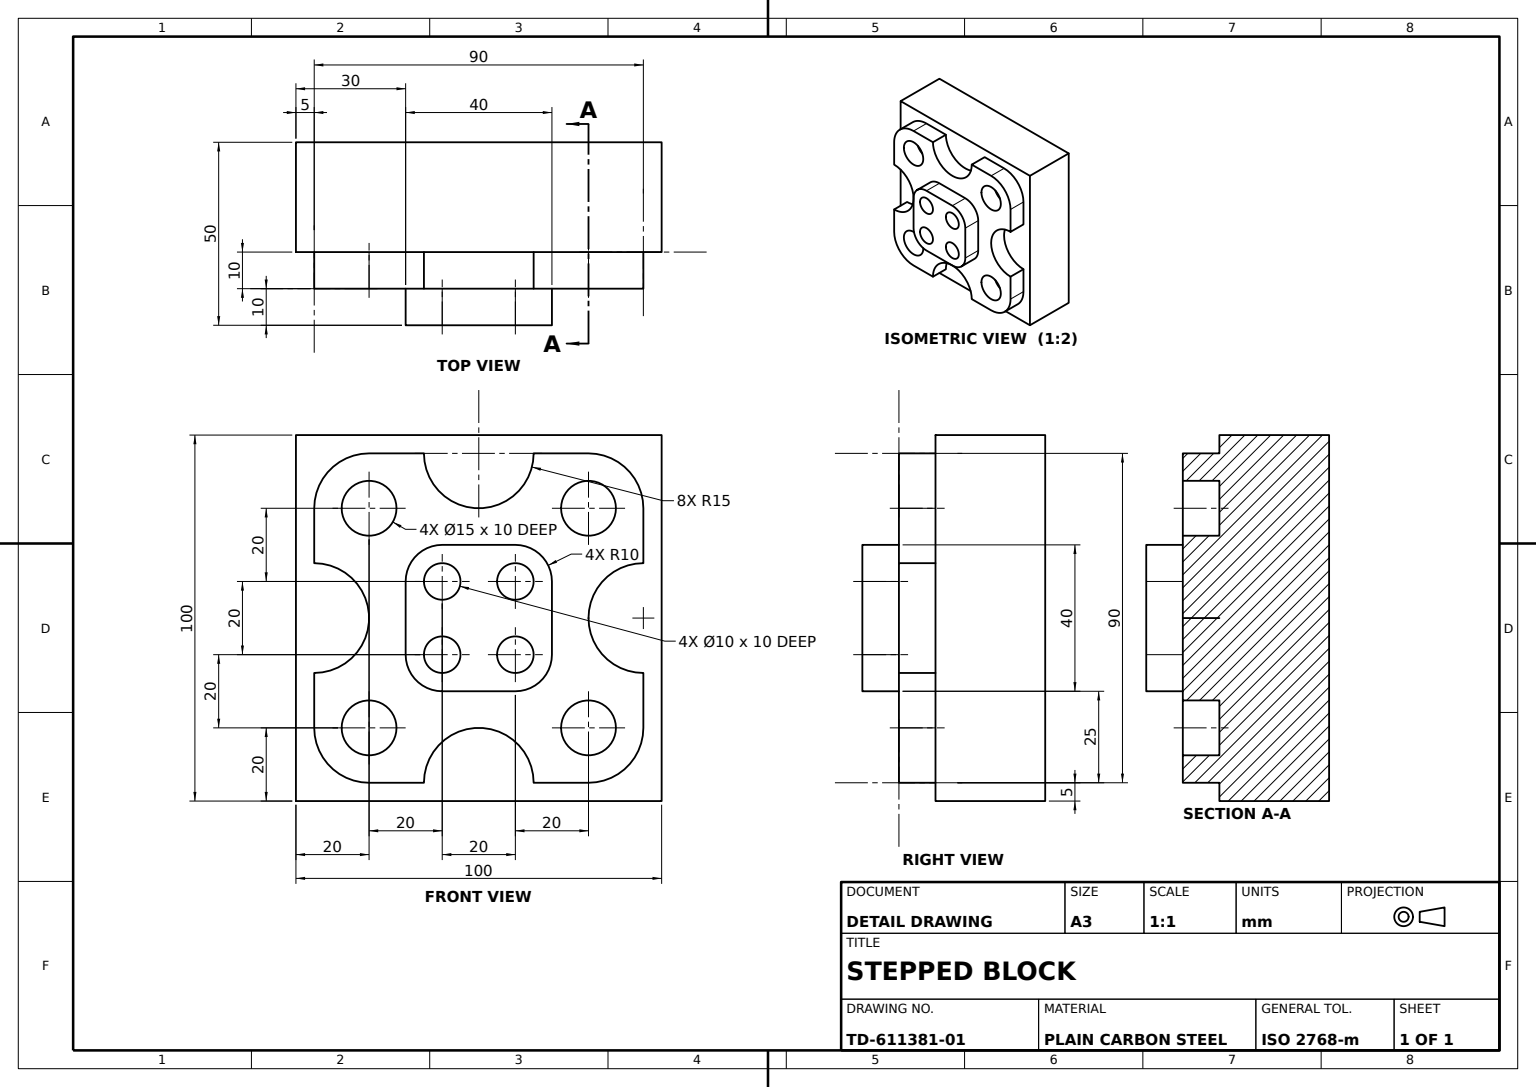
SolidWorks part; units mm, degrees
material "Plain Carbon Steel"
ref_plane "Front Plane" through (0, 0, 0) normal (0, 0, 1) x (1, 0, 0)
ref_plane "Top Plane" through (0, 0, 0) normal (0, 1, 0) x (1, 0, 0)
ref_plane "Right Plane" through (0, 0, 0) normal (1, 0, 0) x (0, 0, -1)
sketch "Base Block Sketch" plane through (0, 0, 0) normal (0, 0, 1) x (1, 0, 0)
  line L0 (50, 45) -> (-50, 45)
  line L1 (50, 0) -> (50, 45)
  line L3 (-50, 45) -> (-50, -55)
  line L4 (-50, -55) -> (50, -55)
  line L5 (50, -55) -> (50, 0)
  dimension "D1" = 100
  dimension "D2" = 100
  dimension "D3" = 50
  dimension "D4" = 45
extrude "Base Block 100x100x30" add sketch "Base Block Sketch" along normal mid plane 30
sketch "Locating Pads Sketch" plane through (0, 0, -15) normal (0, 0, -1) x (-1, 0, 0)
  line L0 (15, 40) -> (45, 40)
  line L2 (45, 40) -> (45, 10)
  line L3 (45, -50) -> (15, -50)
  line L4 (-45, -50) -> (-45, -20)
  line L5 (-45, 40) -> (-15, 40)
  line L6 (-15, -50) -> (-45, -50)
  line L7 (-45, 10) -> (-45, 40)
  line L8 (45, -20) -> (45, -50)
  arc A0 (-45, -20) -> (-45, 10) centre (-45, -5) ccw
  arc A1 (45, 10) -> (45, -20) centre (45, -5) ccw
  arc A2 (-15, 40) -> (15, 40) centre (0, 40) ccw
  arc A3 (15, -50) -> (-15, -50) centre (0, -50) ccw
  dimension "D1" = 15
  dimension "D2" = 15
  dimension "D3" = 15
  dimension "D4" = 15
  dimension "D5" = 40
  dimension "D6" = 50
  dimension "D7" = 90
  dimension "D8" = 5
  dimension "D9" = 5
  dimension "D10" = 45
  dimension "D11" = 45
  dimension "D12" = 45
  dimension "D13" = 90
  dimension "D14" = 45
  dimension "D15" = 45
  dimension "D16" = 40
extrude "Locating Pads 10mm" add sketch "Locating Pads Sketch" along normal blind 10
fillet "Locating Pad Fillet R15 1" radius 15 1 edges at (-45, -50, -20)
fillet "Locating Pad Fillet R15 2" radius 15 1 edges at (45, -50, -20)
fillet "Locating Pad Fillet R15 3" radius 15 1 edges at (45, 40, -20)
fillet "Locating Pad Fillet R15 4" radius 15 1 edges at (-45, 40, -20)
sketch "Raised Pad Sketch" plane through (0, 0, -25) normal (0, 0, -1) x (-1, 0, 0)
  line L0 (50, -55) -> (-50, -55) construction
  line L2 (0, -25) -> (20, -25)
  line L3 (20, -25) -> (20, 15)
  line L4 (20, 15) -> (-20, 15)
  line L5 (-20, 15) -> (-20, -25)
  line L6 (-20, -25) -> (0, -25)
  arc A2 (-45, -20) -> (-45, 10) centre (-45, -5) ccw construction
  arc A3 (15, -50) -> (-15, -50) centre (0, -50) ccw construction
  point P5 (-30, -5)
  dimension "D1" = 40
  dimension "D2" = 40
  dimension "D3" = 70
  dimension "D4" = 50
  dimension "D5" = 25
extrude "Raised Pad 10mm" add sketch "Raised Pad Sketch" along normal blind 10
fillet "Raised Pad Fillet R10 1" radius 10 1 edges at (20, -25, -30)
fillet "Raised Pad Fillet R10 2" radius 10 1 edges at (20, 15, -30)
fillet "Raised Pad Fillet R10 3" radius 10 1 edges at (-20, 15, -30)
fillet "Raised Pad Fillet R10 4" radius 10 1 edges at (-20, -25, -30)
sketch "Raised Pad Pocket Sketch" plane through (0, 0, -35) normal (0, 0, -1) x (-1, 0, 0)
  circle A0 centre (10, 5) radius 5
  circle A1 centre (10, -15) radius 5
  circle A2 centre (-10, -15) radius 5
  circle A3 centre (-10, 5) radius 5
  dimension "D1" = 10
  dimension "D2" = 10
  dimension "D3" = 10
  dimension "D4" = 10
extrude "Raised Pad Pocket 10x10x10" cut sketch "Raised Pad Pocket Sketch" against normal blind 10
sketch "Locating Pad Pocket Sketch" plane through (0, 0, -25) normal (0, 0, -1) x (-1, 0, 0)
  circle A0 centre (30, 25) radius 7.5
  circle A1 centre (30, -35) radius 7.5
  circle A2 centre (-30, -35) radius 7.5
  circle A3 centre (-30, 25) radius 7.5
  dimension "D1" = 15
  dimension "D2" = 15
  dimension "D3" = 15
  dimension "D4" = 15
extrude "Locating Pad Pocket 15x15x10" cut sketch "Locating Pad Pocket Sketch" against normal blind 10
